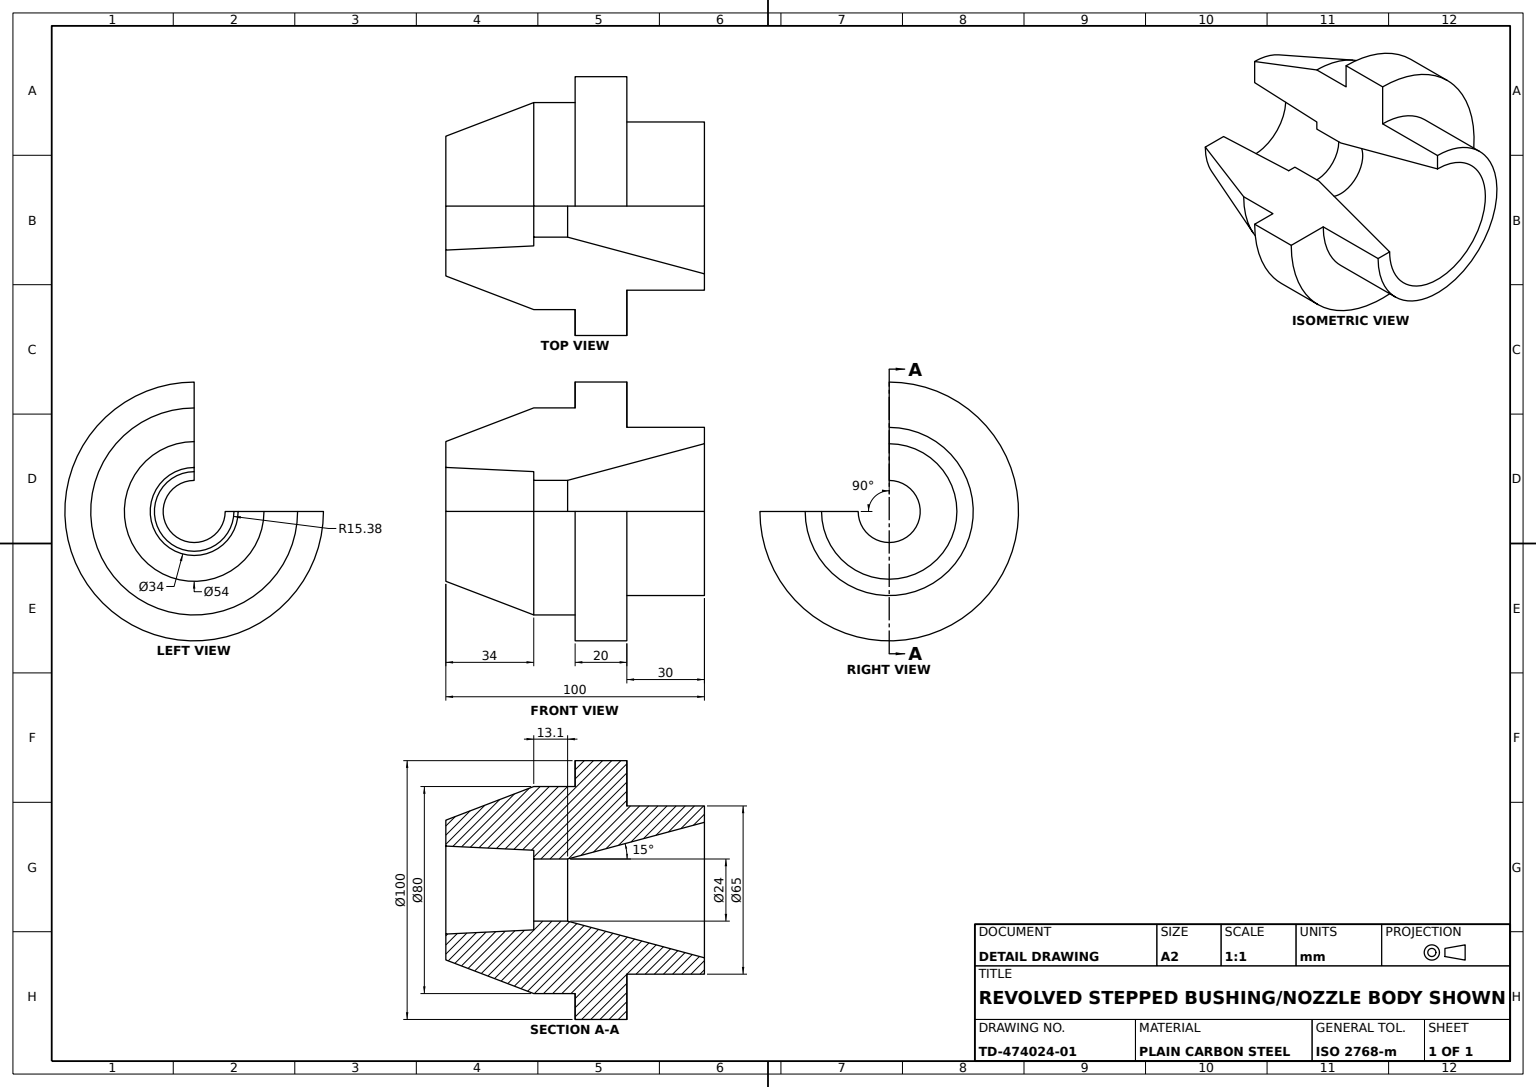
from build123d import *

# Parameters (mm, degrees)
HUB_BODY_REVOLVE_270DEG_ANGLE = 270


with BuildPart() as part:
    # Hub Profile Sketch → Hub Body Revolve 270deg (revolve)
    with BuildSketch(Plane(origin=(0, 0, 0), x_dir=(0, 0, -1), z_dir=(1, 0, 0))):
        Polygon((0, 0), (0, 27), (34, 40), (50, 40), (50, 50), (70, 50), (70, 32.5), (100, 32.5), (100, 0), align=None)
    revolve(axis=Axis((0, 0, -100), (0, 0, 1)), revolution_arc=HUB_BODY_REVOLVE_270DEG_ANGLE)

    # Tapered Bore Profile Sketch → Stepped Tapered Bore Cut (revolve, cut)
    with BuildSketch(Plane(origin=(0, 0, 0), x_dir=(0, 0, -1), z_dir=(1, 0, 0))):
        Polygon((0, 0), (0, 17), (34, 15.380026541), (34, 12), (47.09584733, 12), (100, 26.175624984), (100, 0), align=None)
    revolve(axis=Axis((0, 0, 0), (0, 0, -1)), mode=Mode.SUBTRACT)


solid = part.part
